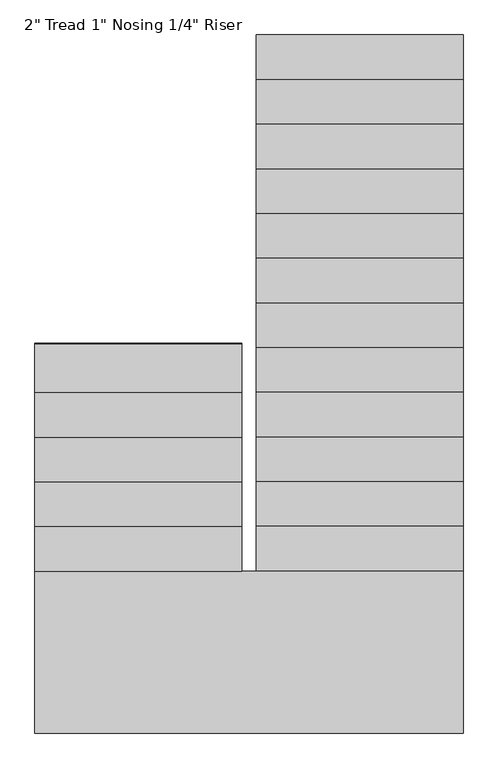
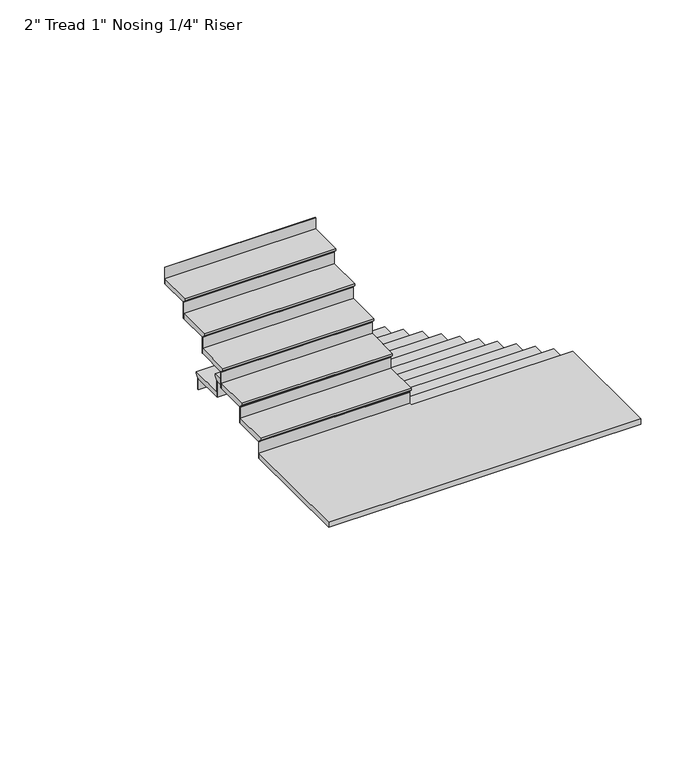
"""IFC4 building model written with IfcOpenShell, lengths in millimetres: stair flight geometry."""

from ifc_helpers import new_model, si_unit, origin, place, context, project, spatial, faceted_brep, source, transform, mapped, element, save


def stair_flight_2e5e19c8(model_context):
    return source(origin(), model_context, "Body", "Brep", [
        faceted_brep([(-1121.360394, -1150.2831508, 6237.3710526), (-1121.360394, -1150.2831508, 6256.4210526), (288.339606, -1150.2831508, 6256.4210526), (288.339606, -1150.2831508, 6237.3710526), (-1121.360394, -1175.6831508, 6211.9710526), (288.339606, -1175.6831508, 6211.9710526), (-1121.360394, -1480.4831508, 6256.4210526), (288.339606, -1480.4831508, 6256.4210526), (288.339606, -1175.6831508, 6205.6210526), (288.339606, -1480.4831508, 6205.6210526), (-1121.360394, -1480.4831508, 6205.6210526), (-1121.360394, -1175.6831508, 6205.6210526)], [[[0, 1, 2, 3]], [[4, 0, 3, 5]], [[2, 1, 6, 7]], [[8, 9, 10, 11]], [[2, 7, 9, 8, 5, 3]], [[8, 11, 4, 5]], [[6, 1, 0, 4, 11, 10]], [[7, 6, 10, 9]]]),
        faceted_brep([(-1121.360394, -1175.6831508, 6205.6210526), (-1121.360394, -1175.6831508, 6096.0), (-1121.360394, -1182.0331508, 6096.0), (-1121.360394, -1182.0331508, 6205.6210526), (288.339606, -1175.6831508, 6205.6210526), (288.339606, -1182.0331508, 6205.6210526), (288.339606, -1182.0331508, 6096.0), (288.339606, -1175.6831508, 6096.0)], [[[0, 1, 2, 3]], [[4, 5, 6, 7]], [[1, 0, 4, 7]], [[2, 1, 7, 6]], [[3, 2, 6, 5]], [[0, 3, 5, 4]]]),
        faceted_brep([(-1121.360394, -1480.4831508, 6366.0421053), (-1121.360394, -1480.4831508, 6205.6210526), (-1121.360394, -1486.8331508, 6205.6210526), (-1121.360394, -1486.8331508, 6366.0421053), (288.339606, -1480.4831508, 6366.0421053), (288.339606, -1486.8331508, 6366.0421053), (288.339606, -1486.8331508, 6205.6210526), (288.339606, -1480.4831508, 6205.6210526)], [[[0, 1, 2, 3]], [[4, 5, 6, 7]], [[1, 0, 4, 7]], [[2, 1, 7, 6]], [[3, 2, 6, 5]], [[0, 3, 5, 4]]]),
        faceted_brep([(288.339606, -1455.0831508, 6416.8421053), (-1121.360394, -1455.0831508, 6416.8421053), (-1121.360394, -1785.2831508, 6416.8421053), (288.339606, -1785.2831508, 6416.8421053), (288.339606, -1480.4831508, 6366.0421053), (288.339606, -1785.2831508, 6366.0421053), (-1121.360394, -1785.2831508, 6366.0421053), (-1121.360394, -1480.4831508, 6366.0421053), (288.339606, -1480.4831508, 6372.3921053), (288.339606, -1455.0831508, 6397.7921053), (-1121.360394, -1480.4831508, 6372.3921053), (-1121.360394, -1455.0831508, 6397.7921053)], [[[0, 1, 2, 3]], [[4, 5, 6, 7]], [[0, 3, 5, 4, 8, 9]], [[4, 7, 10, 8]], [[2, 1, 11, 10, 7, 6]], [[3, 2, 6, 5]], [[11, 1, 0, 9]], [[10, 11, 9, 8]]]),
        faceted_brep([(-1121.360394, -1785.2831508, 6526.4631579), (-1121.360394, -1785.2831508, 6366.0421053), (-1121.360394, -1791.6331508, 6366.0421053), (-1121.360394, -1791.6331508, 6526.4631579), (288.339606, -1785.2831508, 6526.4631579), (288.339606, -1791.6331508, 6526.4631579), (288.339606, -1791.6331508, 6366.0421053), (288.339606, -1785.2831508, 6366.0421053)], [[[0, 1, 2, 3]], [[4, 5, 6, 7]], [[1, 0, 4, 7]], [[2, 1, 7, 6]], [[3, 2, 6, 5]], [[0, 3, 5, 4]]]),
        faceted_brep([(288.339606, -1759.8831508, 6577.2631579), (-1121.360394, -1759.8831508, 6577.2631579), (-1121.360394, -2090.0831508, 6577.2631579), (288.339606, -2090.0831508, 6577.2631579), (288.339606, -1785.2831508, 6526.4631579), (288.339606, -2090.0831508, 6526.4631579), (-1121.360394, -2090.0831508, 6526.4631579), (-1121.360394, -1785.2831508, 6526.4631579), (288.339606, -1785.2831508, 6532.8131579), (288.339606, -1759.8831508, 6558.2131579), (-1121.360394, -1785.2831508, 6532.8131579), (-1121.360394, -1759.8831508, 6558.2131579)], [[[0, 1, 2, 3]], [[4, 5, 6, 7]], [[0, 3, 5, 4, 8, 9]], [[4, 7, 10, 8]], [[2, 1, 11, 10, 7, 6]], [[3, 2, 6, 5]], [[11, 1, 0, 9]], [[10, 11, 9, 8]]]),
        faceted_brep([(-1121.360394, -2090.0831508, 6686.8842105), (-1121.360394, -2090.0831508, 6526.4631579), (-1121.360394, -2096.4331508, 6526.4631579), (-1121.360394, -2096.4331508, 6686.8842105), (288.339606, -2090.0831508, 6686.8842105), (288.339606, -2096.4331508, 6686.8842105), (288.339606, -2096.4331508, 6526.4631579), (288.339606, -2090.0831508, 6526.4631579)], [[[0, 1, 2, 3]], [[4, 5, 6, 7]], [[1, 0, 4, 7]], [[2, 1, 7, 6]], [[3, 2, 6, 5]], [[0, 3, 5, 4]]]),
        faceted_brep([(288.339606, -2064.6831508, 6737.6842105), (-1121.360394, -2064.6831508, 6737.6842105), (-1121.360394, -2394.8831508, 6737.6842105), (288.339606, -2394.8831508, 6737.6842105), (288.339606, -2090.0831508, 6686.8842105), (288.339606, -2394.8831508, 6686.8842105), (-1121.360394, -2394.8831508, 6686.8842105), (-1121.360394, -2090.0831508, 6686.8842105), (288.339606, -2090.0831508, 6693.2342105), (288.339606, -2064.6831508, 6718.6342105), (-1121.360394, -2090.0831508, 6693.2342105), (-1121.360394, -2064.6831508, 6718.6342105)], [[[0, 1, 2, 3]], [[4, 5, 6, 7]], [[0, 3, 5, 4, 8, 9]], [[4, 7, 10, 8]], [[2, 1, 11, 10, 7, 6]], [[3, 2, 6, 5]], [[11, 1, 0, 9]], [[10, 11, 9, 8]]]),
        faceted_brep([(-1121.360394, -2394.8831508, 6847.3052632), (-1121.360394, -2394.8831508, 6686.8842105), (-1121.360394, -2401.2331508, 6686.8842105), (-1121.360394, -2401.2331508, 6847.3052632), (288.339606, -2394.8831508, 6847.3052632), (288.339606, -2401.2331508, 6847.3052632), (288.339606, -2401.2331508, 6686.8842105), (288.339606, -2394.8831508, 6686.8842105)], [[[0, 1, 2, 3]], [[4, 5, 6, 7]], [[1, 0, 4, 7]], [[2, 1, 7, 6]], [[3, 2, 6, 5]], [[0, 3, 5, 4]]]),
        faceted_brep([(288.339606, -2369.4831508, 6898.1052632), (-1121.360394, -2369.4831508, 6898.1052632), (-1121.360394, -2699.6831508, 6898.1052632), (288.339606, -2699.6831508, 6898.1052632), (288.339606, -2394.8831508, 6847.3052632), (288.339606, -2699.6831508, 6847.3052632), (-1121.360394, -2699.6831508, 6847.3052632), (-1121.360394, -2394.8831508, 6847.3052632), (288.339606, -2394.8831508, 6853.6552632), (288.339606, -2369.4831508, 6879.0552632), (-1121.360394, -2394.8831508, 6853.6552632), (-1121.360394, -2369.4831508, 6879.0552632)], [[[0, 1, 2, 3]], [[4, 5, 6, 7]], [[0, 3, 5, 4, 8, 9]], [[4, 7, 10, 8]], [[2, 1, 11, 10, 7, 6]], [[3, 2, 6, 5]], [[11, 1, 0, 9]], [[10, 11, 9, 8]]]),
        faceted_brep([(-1121.360394, -2699.6831508, 7007.7263158), (-1121.360394, -2699.6831508, 6847.3052632), (-1121.360394, -2706.0331508, 6847.3052632), (-1121.360394, -2706.0331508, 7007.7263158), (288.339606, -2699.6831508, 7007.7263158), (288.339606, -2706.0331508, 7007.7263158), (288.339606, -2706.0331508, 6847.3052632), (288.339606, -2699.6831508, 6847.3052632)], [[[0, 1, 2, 3]], [[4, 5, 6, 7]], [[1, 0, 4, 7]], [[2, 1, 7, 6]], [[3, 2, 6, 5]], [[0, 3, 5, 4]]]),
        faceted_brep([(288.339606, -2674.2831508, 7058.5263158), (-1121.360394, -2674.2831508, 7058.5263158), (-1121.360394, -3004.4831508, 7058.5263158), (288.339606, -3004.4831508, 7058.5263158), (288.339606, -2699.6831508, 7007.7263158), (288.339606, -3004.4831508, 7007.7263158), (-1121.360394, -3004.4831508, 7007.7263158), (-1121.360394, -2699.6831508, 7007.7263158), (288.339606, -2699.6831508, 7014.0763158), (288.339606, -2674.2831508, 7039.4763158), (-1121.360394, -2699.6831508, 7014.0763158), (-1121.360394, -2674.2831508, 7039.4763158)], [[[0, 1, 2, 3]], [[4, 5, 6, 7]], [[0, 3, 5, 4, 8, 9]], [[4, 7, 10, 8]], [[2, 1, 11, 10, 7, 6]], [[3, 2, 6, 5]], [[11, 1, 0, 9]], [[10, 11, 9, 8]]]),
        faceted_brep([(-1121.360394, -3004.4831508, 7168.1473684), (-1121.360394, -3004.4831508, 7007.7263158), (-1121.360394, -3010.8331508, 7007.7263158), (-1121.360394, -3010.8331508, 7168.1473684), (288.339606, -3004.4831508, 7168.1473684), (288.339606, -3010.8331508, 7168.1473684), (288.339606, -3010.8331508, 7007.7263158), (288.339606, -3004.4831508, 7007.7263158)], [[[0, 1, 2, 3]], [[4, 5, 6, 7]], [[1, 0, 4, 7]], [[2, 1, 7, 6]], [[3, 2, 6, 5]], [[0, 3, 5, 4]]]),
        faceted_brep([(288.339606, -2979.0831508, 7218.9473684), (-1121.360394, -2979.0831508, 7218.9473684), (-1121.360394, -3309.2831508, 7218.9473684), (288.339606, -3309.2831508, 7218.9473684), (288.339606, -3004.4831508, 7168.1473684), (288.339606, -3309.2831508, 7168.1473684), (-1121.360394, -3309.2831508, 7168.1473684), (-1121.360394, -3004.4831508, 7168.1473684), (288.339606, -3004.4831508, 7174.4973684), (288.339606, -2979.0831508, 7199.8973684), (-1121.360394, -3004.4831508, 7174.4973684), (-1121.360394, -2979.0831508, 7199.8973684)], [[[0, 1, 2, 3]], [[4, 5, 6, 7]], [[0, 3, 5, 4, 8, 9]], [[4, 7, 10, 8]], [[2, 1, 11, 10, 7, 6]], [[3, 2, 6, 5]], [[11, 1, 0, 9]], [[10, 11, 9, 8]]]),
        faceted_brep([(-1121.360394, -3309.2831508, 7328.5684211), (-1121.360394, -3309.2831508, 7168.1473684), (-1121.360394, -3315.6331508, 7168.1473684), (-1121.360394, -3315.6331508, 7328.5684211), (288.339606, -3309.2831508, 7328.5684211), (288.339606, -3315.6331508, 7328.5684211), (288.339606, -3315.6331508, 7168.1473684), (288.339606, -3309.2831508, 7168.1473684)], [[[0, 1, 2, 3]], [[4, 5, 6, 7]], [[1, 0, 4, 7]], [[2, 1, 7, 6]], [[3, 2, 6, 5]], [[0, 3, 5, 4]]]),
        faceted_brep([(288.339606, -3283.8831508, 7379.3684211), (-1121.360394, -3283.8831508, 7379.3684211), (-1121.360394, -3614.0831508, 7379.3684211), (288.339606, -3614.0831508, 7379.3684211), (288.339606, -3309.2831508, 7328.5684211), (288.339606, -3614.0831508, 7328.5684211), (-1121.360394, -3614.0831508, 7328.5684211), (-1121.360394, -3309.2831508, 7328.5684211), (288.339606, -3309.2831508, 7334.9184211), (288.339606, -3283.8831508, 7360.3184211), (-1121.360394, -3309.2831508, 7334.9184211), (-1121.360394, -3283.8831508, 7360.3184211)], [[[0, 1, 2, 3]], [[4, 5, 6, 7]], [[0, 3, 5, 4, 8, 9]], [[4, 7, 10, 8]], [[2, 1, 11, 10, 7, 6]], [[3, 2, 6, 5]], [[11, 1, 0, 9]], [[10, 11, 9, 8]]]),
        faceted_brep([(-1121.360394, -3614.0831508, 7488.9894737), (-1121.360394, -3614.0831508, 7328.5684211), (-1121.360394, -3620.4331508, 7328.5684211), (-1121.360394, -3620.4331508, 7488.9894737), (288.339606, -3614.0831508, 7488.9894737), (288.339606, -3620.4331508, 7488.9894737), (288.339606, -3620.4331508, 7328.5684211), (288.339606, -3614.0831508, 7328.5684211)], [[[0, 1, 2, 3]], [[4, 5, 6, 7]], [[1, 0, 4, 7]], [[2, 1, 7, 6]], [[3, 2, 6, 5]], [[0, 3, 5, 4]]]),
        faceted_brep([(288.339606, -3588.6831508, 7539.7894737), (-1121.360394, -3588.6831508, 7539.7894737), (-1121.360394, -3918.8831508, 7539.7894737), (288.339606, -3918.8831508, 7539.7894737), (288.339606, -3614.0831508, 7488.9894737), (288.339606, -3918.8831508, 7488.9894737), (-1121.360394, -3918.8831508, 7488.9894737), (-1121.360394, -3614.0831508, 7488.9894737), (288.339606, -3614.0831508, 7495.3394737), (288.339606, -3588.6831508, 7520.7394737), (-1121.360394, -3614.0831508, 7495.3394737), (-1121.360394, -3588.6831508, 7520.7394737)], [[[0, 1, 2, 3]], [[4, 5, 6, 7]], [[0, 3, 5, 4, 8, 9]], [[4, 7, 10, 8]], [[2, 1, 11, 10, 7, 6]], [[3, 2, 6, 5]], [[11, 1, 0, 9]], [[10, 11, 9, 8]]]),
        faceted_brep([(-1121.360394, -3918.8831508, 7649.4105263), (-1121.360394, -3918.8831508, 7488.9894737), (-1121.360394, -3925.2331508, 7488.9894737), (-1121.360394, -3925.2331508, 7649.4105263), (288.339606, -3918.8831508, 7649.4105263), (288.339606, -3925.2331508, 7649.4105263), (288.339606, -3925.2331508, 7488.9894737), (288.339606, -3918.8831508, 7488.9894737)], [[[0, 1, 2, 3]], [[4, 5, 6, 7]], [[1, 0, 4, 7]], [[2, 1, 7, 6]], [[3, 2, 6, 5]], [[0, 3, 5, 4]]]),
        faceted_brep([(288.339606, -3893.4831508, 7700.2105263), (-1121.360394, -3893.4831508, 7700.2105263), (-1121.360394, -4223.6831508, 7700.2105263), (288.339606, -4223.6831508, 7700.2105263), (288.339606, -3918.8831508, 7649.4105263), (288.339606, -4223.6831508, 7649.4105263), (-1121.360394, -4223.6831508, 7649.4105263), (-1121.360394, -3918.8831508, 7649.4105263), (288.339606, -3918.8831508, 7655.7605263), (288.339606, -3893.4831508, 7681.1605263), (-1121.360394, -3918.8831508, 7655.7605263), (-1121.360394, -3893.4831508, 7681.1605263)], [[[0, 1, 2, 3]], [[4, 5, 6, 7]], [[0, 3, 5, 4, 8, 9]], [[4, 7, 10, 8]], [[2, 1, 11, 10, 7, 6]], [[3, 2, 6, 5]], [[11, 1, 0, 9]], [[10, 11, 9, 8]]]),
        faceted_brep([(-1121.360394, -4223.6831508, 7809.8315789), (-1121.360394, -4223.6831508, 7649.4105263), (-1121.360394, -4230.0331508, 7649.4105263), (-1121.360394, -4230.0331508, 7809.8315789), (288.339606, -4223.6831508, 7809.8315789), (288.339606, -4230.0331508, 7809.8315789), (288.339606, -4230.0331508, 7649.4105263), (288.339606, -4223.6831508, 7649.4105263)], [[[0, 1, 2, 3]], [[4, 5, 6, 7]], [[1, 0, 4, 7]], [[2, 1, 7, 6]], [[3, 2, 6, 5]], [[0, 3, 5, 4]]]),
        faceted_brep([(288.339606, -4198.2831508, 7860.6315789), (-1121.360394, -4198.2831508, 7860.6315789), (-1121.360394, -4528.4831508, 7860.6315789), (288.339606, -4528.4831508, 7860.6315789), (288.339606, -4223.6831508, 7809.8315789), (288.339606, -4528.4831508, 7809.8315789), (-1121.360394, -4528.4831508, 7809.8315789), (-1121.360394, -4223.6831508, 7809.8315789), (288.339606, -4223.6831508, 7816.1815789), (288.339606, -4198.2831508, 7841.5815789), (-1121.360394, -4223.6831508, 7816.1815789), (-1121.360394, -4198.2831508, 7841.5815789)], [[[0, 1, 2, 3]], [[4, 5, 6, 7]], [[0, 3, 5, 4, 8, 9]], [[4, 7, 10, 8]], [[2, 1, 11, 10, 7, 6]], [[3, 2, 6, 5]], [[11, 1, 0, 9]], [[10, 11, 9, 8]]]),
        faceted_brep([(-1121.360394, -4528.4831508, 7970.2526316), (-1121.360394, -4528.4831508, 7809.8315789), (-1121.360394, -4534.8331508, 7809.8315789), (-1121.360394, -4534.8331508, 7970.2526316), (288.339606, -4528.4831508, 7970.2526316), (288.339606, -4534.8331508, 7970.2526316), (288.339606, -4534.8331508, 7809.8315789), (288.339606, -4528.4831508, 7809.8315789)], [[[0, 1, 2, 3]], [[4, 5, 6, 7]], [[1, 0, 4, 7]], [[2, 1, 7, 6]], [[3, 2, 6, 5]], [[0, 3, 5, 4]]]),
        faceted_brep([(288.339606, -4503.0831508, 8021.0526316), (-1121.360394, -4503.0831508, 8021.0526316), (-1121.360394, -4833.2831508, 8021.0526316), (288.339606, -4833.2831508, 8021.0526316), (288.339606, -4528.4831508, 7970.2526316), (288.339606, -4833.2831508, 7970.2526316), (-1121.360394, -4833.2831508, 7970.2526316), (-1121.360394, -4528.4831508, 7970.2526316), (288.339606, -4528.4831508, 7976.6026316), (288.339606, -4503.0831508, 8002.0026316), (-1121.360394, -4528.4831508, 7976.6026316), (-1121.360394, -4503.0831508, 8002.0026316)], [[[0, 1, 2, 3]], [[4, 5, 6, 7]], [[0, 3, 5, 4, 8, 9]], [[4, 7, 10, 8]], [[2, 1, 11, 10, 7, 6]], [[3, 2, 6, 5]], [[11, 1, 0, 9]], [[10, 11, 9, 8]]]),
        faceted_brep([(-1121.360394, -4833.2831508, 8130.6736842), (-1121.360394, -4833.2831508, 7970.2526316), (-1121.360394, -4839.6331508, 7970.2526316), (-1121.360394, -4839.6331508, 8130.6736842), (288.339606, -4833.2831508, 8130.6736842), (288.339606, -4839.6331508, 8130.6736842), (288.339606, -4839.6331508, 7970.2526316), (288.339606, -4833.2831508, 7970.2526316)], [[[0, 1, 2, 3]], [[4, 5, 6, 7]], [[1, 0, 4, 7]], [[2, 1, 7, 6]], [[3, 2, 6, 5]], [[0, 3, 5, 4]]]),
        faceted_brep([(-2632.660394, -4782.4831508, 8181.4736842), (-2632.660394, -5912.7831508, 8181.4736842), (288.339606, -5912.7831508, 8181.4736842), (288.339606, -4807.8831508, 8181.4736842), (-1222.960394, -4807.8831508, 8181.4736842), (-1222.960394, -4782.4831508, 8181.4736842), (-2632.660394, -5912.7831508, 8130.6736842), (-2632.660394, -4782.4831508, 8130.6736842), (-1222.960394, -4782.4831508, 8130.6736842), (-1222.960394, -4807.8831508, 8130.6736842), (-1121.360394, -4807.8831508, 8130.6736842), (-1121.360394, -4833.2831508, 8130.6736842), (288.339606, -4833.2831508, 8130.6736842), (288.339606, -5912.7831508, 8130.6736842), (288.339606, -4833.2831508, 8137.0236842), (288.339606, -4807.8831508, 8162.4236842), (-1121.360394, -4833.2831508, 8137.0236842), (-1121.360394, -4807.8831508, 8162.4236842)], [[[0, 1, 2, 3, 4, 5]], [[6, 7, 8, 9, 10, 11, 12, 13]], [[1, 0, 7, 6]], [[2, 1, 6, 13]], [[3, 2, 13, 12, 14, 15]], [[12, 11, 16, 14]], [[11, 10, 17, 16]], [[4, 3, 15, 17, 10, 9]], [[5, 4, 9, 8]], [[0, 5, 8, 7]], [[15, 14, 16, 17]]]),
        faceted_brep([(-1222.960394, -4782.4831508, 8291.0947368), (-1222.960394, -4782.4831508, 8130.6736842), (-1222.960394, -4776.1331508, 8130.6736842), (-1222.960394, -4776.1331508, 8291.0947368), (-2632.660394, -4782.4831508, 8291.0947368), (-2632.660394, -4776.1331508, 8291.0947368), (-2632.660394, -4776.1331508, 8130.6736842), (-2632.660394, -4782.4831508, 8130.6736842)], [[[0, 1, 2, 3]], [[4, 5, 6, 7]], [[1, 0, 4, 7]], [[2, 1, 7, 6]], [[3, 2, 6, 5]], [[0, 3, 5, 4]]]),
        faceted_brep([(-2632.660394, -4807.8831508, 8341.8947368), (-1222.960394, -4807.8831508, 8341.8947368), (-1222.960394, -4477.6831508, 8341.8947368), (-2632.660394, -4477.6831508, 8341.8947368), (-2632.660394, -4782.4831508, 8291.0947368), (-2632.660394, -4477.6831508, 8291.0947368), (-1222.960394, -4477.6831508, 8291.0947368), (-1222.960394, -4782.4831508, 8291.0947368), (-2632.660394, -4782.4831508, 8297.4447368), (-2632.660394, -4807.8831508, 8322.8447368), (-1222.960394, -4782.4831508, 8297.4447368), (-1222.960394, -4807.8831508, 8322.8447368)], [[[0, 1, 2, 3]], [[4, 5, 6, 7]], [[0, 3, 5, 4, 8, 9]], [[4, 7, 10, 8]], [[2, 1, 11, 10, 7, 6]], [[3, 2, 6, 5]], [[11, 1, 0, 9]], [[10, 11, 9, 8]]]),
        faceted_brep([(-1222.960394, -4477.6831508, 8451.5157895), (-1222.960394, -4477.6831508, 8291.0947368), (-1222.960394, -4471.3331508, 8291.0947368), (-1222.960394, -4471.3331508, 8451.5157895), (-2632.660394, -4477.6831508, 8451.5157895), (-2632.660394, -4471.3331508, 8451.5157895), (-2632.660394, -4471.3331508, 8291.0947368), (-2632.660394, -4477.6831508, 8291.0947368)], [[[0, 1, 2, 3]], [[4, 5, 6, 7]], [[1, 0, 4, 7]], [[2, 1, 7, 6]], [[3, 2, 6, 5]], [[0, 3, 5, 4]]]),
        faceted_brep([(-2632.660394, -4503.0831508, 8502.3157895), (-1222.960394, -4503.0831508, 8502.3157895), (-1222.960394, -4172.8831508, 8502.3157895), (-2632.660394, -4172.8831508, 8502.3157895), (-2632.660394, -4477.6831508, 8451.5157895), (-2632.660394, -4172.8831508, 8451.5157895), (-1222.960394, -4172.8831508, 8451.5157895), (-1222.960394, -4477.6831508, 8451.5157895), (-2632.660394, -4477.6831508, 8457.8657895), (-2632.660394, -4503.0831508, 8483.2657895), (-1222.960394, -4477.6831508, 8457.8657895), (-1222.960394, -4503.0831508, 8483.2657895)], [[[0, 1, 2, 3]], [[4, 5, 6, 7]], [[0, 3, 5, 4, 8, 9]], [[4, 7, 10, 8]], [[2, 1, 11, 10, 7, 6]], [[3, 2, 6, 5]], [[11, 1, 0, 9]], [[10, 11, 9, 8]]]),
        faceted_brep([(-1222.960394, -4172.8831508, 8611.9368421), (-1222.960394, -4172.8831508, 8451.5157895), (-1222.960394, -4166.5331508, 8451.5157895), (-1222.960394, -4166.5331508, 8611.9368421), (-2632.660394, -4172.8831508, 8611.9368421), (-2632.660394, -4166.5331508, 8611.9368421), (-2632.660394, -4166.5331508, 8451.5157895), (-2632.660394, -4172.8831508, 8451.5157895)], [[[0, 1, 2, 3]], [[4, 5, 6, 7]], [[1, 0, 4, 7]], [[2, 1, 7, 6]], [[3, 2, 6, 5]], [[0, 3, 5, 4]]]),
        faceted_brep([(-2632.660394, -4198.2831508, 8662.7368421), (-1222.960394, -4198.2831508, 8662.7368421), (-1222.960394, -3868.0831508, 8662.7368421), (-2632.660394, -3868.0831508, 8662.7368421), (-2632.660394, -4172.8831508, 8611.9368421), (-2632.660394, -3868.0831508, 8611.9368421), (-1222.960394, -3868.0831508, 8611.9368421), (-1222.960394, -4172.8831508, 8611.9368421), (-2632.660394, -4172.8831508, 8618.2868421), (-2632.660394, -4198.2831508, 8643.6868421), (-1222.960394, -4172.8831508, 8618.2868421), (-1222.960394, -4198.2831508, 8643.6868421)], [[[0, 1, 2, 3]], [[4, 5, 6, 7]], [[0, 3, 5, 4, 8, 9]], [[4, 7, 10, 8]], [[2, 1, 11, 10, 7, 6]], [[3, 2, 6, 5]], [[11, 1, 0, 9]], [[10, 11, 9, 8]]]),
        faceted_brep([(-1222.960394, -3868.0831508, 8772.3578947), (-1222.960394, -3868.0831508, 8611.9368421), (-1222.960394, -3861.7331508, 8611.9368421), (-1222.960394, -3861.7331508, 8772.3578947), (-2632.660394, -3868.0831508, 8772.3578947), (-2632.660394, -3861.7331508, 8772.3578947), (-2632.660394, -3861.7331508, 8611.9368421), (-2632.660394, -3868.0831508, 8611.9368421)], [[[0, 1, 2, 3]], [[4, 5, 6, 7]], [[1, 0, 4, 7]], [[2, 1, 7, 6]], [[3, 2, 6, 5]], [[0, 3, 5, 4]]]),
        faceted_brep([(-2632.660394, -3893.4831508, 8823.1578947), (-1222.960394, -3893.4831508, 8823.1578947), (-1222.960394, -3563.2831508, 8823.1578947), (-2632.660394, -3563.2831508, 8823.1578947), (-2632.660394, -3868.0831508, 8772.3578947), (-2632.660394, -3563.2831508, 8772.3578947), (-1222.960394, -3563.2831508, 8772.3578947), (-1222.960394, -3868.0831508, 8772.3578947), (-2632.660394, -3868.0831508, 8778.7078947), (-2632.660394, -3893.4831508, 8804.1078947), (-1222.960394, -3868.0831508, 8778.7078947), (-1222.960394, -3893.4831508, 8804.1078947)], [[[0, 1, 2, 3]], [[4, 5, 6, 7]], [[0, 3, 5, 4, 8, 9]], [[4, 7, 10, 8]], [[2, 1, 11, 10, 7, 6]], [[3, 2, 6, 5]], [[11, 1, 0, 9]], [[10, 11, 9, 8]]]),
        faceted_brep([(-1222.960394, -3563.2831508, 8932.7789474), (-1222.960394, -3563.2831508, 8772.3578947), (-1222.960394, -3556.9331508, 8772.3578947), (-1222.960394, -3556.9331508, 8932.7789474), (-2632.660394, -3563.2831508, 8932.7789474), (-2632.660394, -3556.9331508, 8932.7789474), (-2632.660394, -3556.9331508, 8772.3578947), (-2632.660394, -3563.2831508, 8772.3578947)], [[[0, 1, 2, 3]], [[4, 5, 6, 7]], [[1, 0, 4, 7]], [[2, 1, 7, 6]], [[3, 2, 6, 5]], [[0, 3, 5, 4]]]),
        faceted_brep([(-1222.960394, -3258.4831508, 9093.2), (-1222.960394, -3258.4831508, 8932.7789474), (-1222.960394, -3252.1331508, 8932.7789474), (-1222.960394, -3252.1331508, 9093.2), (-2632.660394, -3258.4831508, 9093.2), (-2632.660394, -3252.1331508, 9093.2), (-2632.660394, -3252.1331508, 8932.7789474), (-2632.660394, -3258.4831508, 8932.7789474)], [[[0, 1, 2, 3]], [[4, 5, 6, 7]], [[1, 0, 4, 7]], [[2, 1, 7, 6]], [[3, 2, 6, 5]], [[0, 3, 5, 4]]]),
        faceted_brep([(-2632.660394, -3588.6831508, 8983.5789474), (-1222.960394, -3588.6831508, 8983.5789474), (-1222.960394, -3258.4831508, 8983.5789474), (-2632.660394, -3258.4831508, 8983.5789474), (-2632.660394, -3563.2831508, 8932.7789474), (-2632.660394, -3258.4831508, 8932.7789474), (-1222.960394, -3258.4831508, 8932.7789474), (-1222.960394, -3563.2831508, 8932.7789474), (-2632.660394, -3563.2831508, 8939.1289474), (-2632.660394, -3588.6831508, 8964.5289474), (-1222.960394, -3563.2831508, 8939.1289474), (-1222.960394, -3588.6831508, 8964.5289474)], [[[0, 1, 2, 3]], [[4, 5, 6, 7]], [[0, 3, 5, 4, 8, 9]], [[4, 7, 10, 8]], [[2, 1, 11, 10, 7, 6]], [[3, 2, 6, 5]], [[11, 1, 0, 9]], [[10, 11, 9, 8]]]),
    ])


if __name__ == "__main__":
    model = new_model("IFC4")
    model_context = context("Model", 3, world=origin())
    ifc_project = project(units=[si_unit("LENGTHUNIT", "METRE", prefix="MILLI")], contexts=[model_context])
    site = spatial("IfcSite", under=ifc_project)
    building = spatial("IfcBuilding", under=site)
    placement = place(None, origin())
    stair_flight_shape = stair_flight_2e5e19c8(model_context)
    element("IfcStairFlight", 1, ObjectType="2\" Tread 1\" Nosing 1/4\" Riser", at=placement, inside=building, context=model_context, shape_type="MappedRepresentation", body=[
        mapped(stair_flight_shape, transform((0.0, 0.0, 0.0), x_axis=(1.0, 0.0, 0.0), y_axis=(0.0, 1.0, 0.0), z_axis=(0.0, 0.0, 1.0))),
    ])
    save(model, "model.ifc")
